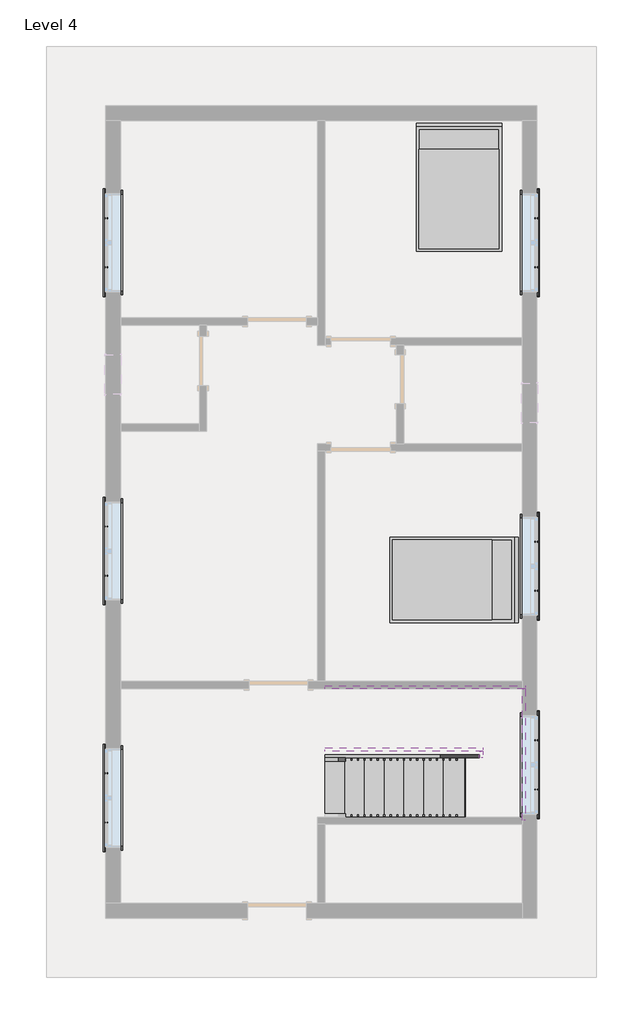
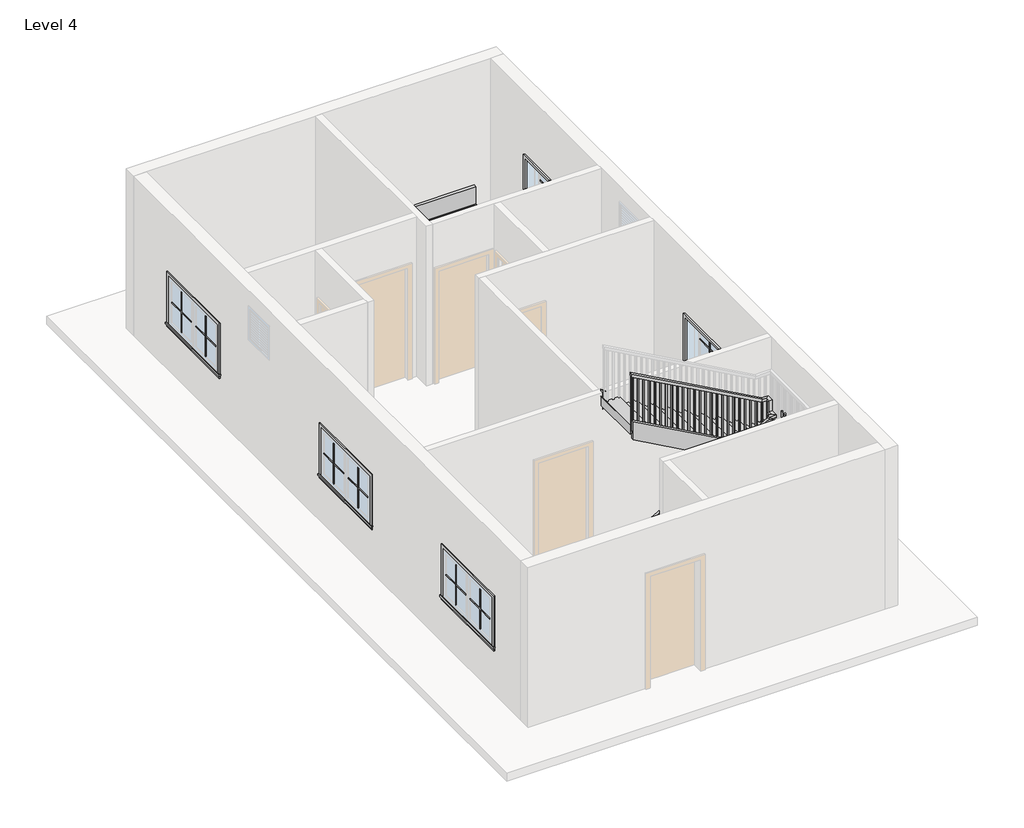
# One storey, part 3 of 3: 24 proxies, 6 members, 2 furniture elements, 1 railing, 1 stair flight.
"""IFC4 building model written with IfcOpenShell, lengths in millimetres."""

from ifc_helpers import new_model, si_unit, frame, origin, place, context, project, spatial, polyline, outline, extrude, faceted_brep, transform, mapped, element, save
from components import muntin_pattern_2x2_muntin_pattern_2x2_9352d081, muntin_pattern_2x2_muntin_pattern_2x2_5c2cbe28, trim_window_exterior_flat_with_sill_979bde60, trim_window_interior_flat_picture_frame_7883d11b, bed_17739_bed_17739_15c61121, stair_flight_ebc403c3

model = new_model("IFC4")

# Units and contexts
model_context = context("Model", 3, world=origin())
ifc_project = project(units=[si_unit("LENGTHUNIT", "METRE", prefix="MILLI")], contexts=[model_context])

# Site, building, storey
site = spatial("IfcSite", under=ifc_project)
building = spatial("IfcBuilding", under=site)
storey = spatial("IfcBuildingStorey", under=building, Name="Level 4", Elevation=9448.8)

# Proxies
placement = place(None, origin())
muntin_pattern_2x2_muntin_pattern_2x2_shape = muntin_pattern_2x2_muntin_pattern_2x2_9352d081(model_context)
element("IfcBuildingElementProxy", 1, Name="Muntin Pattern_2x2 : Muntin Pattern_2x2", ObjectType="Muntin Pattern_2x2 : Muntin Pattern_2x2", at=placement, inside=storey, context=model_context, shape_type="MappedRepresentation", body=[
    mapped(muntin_pattern_2x2_muntin_pattern_2x2_shape, transform((-4579.34688, 3675.02881, 10433.05), x_axis=(0.0, 1.0, 0.0), y_axis=(-1.0, 0.0, 0.0), z_axis=(0.0, 0.0, 1.0))),
])
element("IfcBuildingElementProxy", 2, Name="Muntin Pattern_2x2 : Muntin Pattern_2x2", ObjectType="Muntin Pattern_2x2 : Muntin Pattern_2x2", at=placement, inside=storey, context=model_context, shape_type="MappedRepresentation", body=[
    mapped(muntin_pattern_2x2_muntin_pattern_2x2_shape, transform((-4579.34688, -1087.47119, 10433.05), x_axis=(0.0, 1.0, 0.0), y_axis=(-1.0, 0.0, 0.0), z_axis=(0.0, 0.0, 1.0))),
])
element("IfcBuildingElementProxy", 3, Name="Muntin Pattern_2x2 : Muntin Pattern_2x2", ObjectType="Muntin Pattern_2x2 : Muntin Pattern_2x2", at=placement, inside=storey, context=model_context, shape_type="MappedRepresentation", body=[
    mapped(muntin_pattern_2x2_muntin_pattern_2x2_shape, transform((-4579.34688, -4900.64619, 10433.05), x_axis=(0.0, 1.0, 0.0), y_axis=(-1.0, 0.0, 0.0), z_axis=(0.0, 0.0, 1.0))),
])
element("IfcBuildingElementProxy", 4, Name="Muntin Pattern_2x2 : Muntin Pattern_2x2", ObjectType="Muntin Pattern_2x2 : Muntin Pattern_2x2", at=placement, inside=storey, context=model_context, shape_type="MappedRepresentation", body=[
    mapped(muntin_pattern_2x2_muntin_pattern_2x2_shape, transform((2069.10312, -3630.64619, 10433.05), x_axis=(0.0, -1.0, 0.0), y_axis=(1.0, 0.0, 0.0), z_axis=(0.0, 0.0, 1.0))),
])
element("IfcBuildingElementProxy", 5, Name="Muntin Pattern_2x2 : Muntin Pattern_2x2", ObjectType="Muntin Pattern_2x2 : Muntin Pattern_2x2", at=placement, inside=storey, context=model_context, shape_type="MappedRepresentation", body=[
    mapped(muntin_pattern_2x2_muntin_pattern_2x2_shape, transform((2069.10312, 4433.85381, 10433.05), x_axis=(0.0, -1.0, 0.0), y_axis=(1.0, 0.0, 0.0), z_axis=(0.0, 0.0, 1.0))),
])
element("IfcBuildingElementProxy", 6, Name="Muntin Pattern_2x2 : Muntin Pattern_2x2", ObjectType="Muntin Pattern_2x2 : Muntin Pattern_2x2", at=placement, inside=storey, context=model_context, shape_type="MappedRepresentation", body=[
    mapped(muntin_pattern_2x2_muntin_pattern_2x2_shape, transform((2069.10312, -563.59619, 10433.05), x_axis=(0.0, -1.0, 0.0), y_axis=(1.0, 0.0, 0.0), z_axis=(0.0, 0.0, 1.0))),
])
muntin_pattern_2x2_muntin_pattern_2x2_2_shape = muntin_pattern_2x2_muntin_pattern_2x2_5c2cbe28(model_context)
element("IfcBuildingElementProxy", 7, Name="Muntin Pattern_2x2 : Muntin Pattern_2x2", ObjectType="Muntin Pattern_2x2 : Muntin Pattern_2x2", at=placement, inside=storey, context=model_context, shape_type="MappedRepresentation", body=[
    mapped(muntin_pattern_2x2_muntin_pattern_2x2_2_shape, transform((-4579.34688, 4433.85381, 10433.05), x_axis=(0.0, -1.0, 0.0), y_axis=(1.0, 0.0, 0.0), z_axis=(0.0, 0.0, 1.0))),
])
element("IfcBuildingElementProxy", 8, Name="Muntin Pattern_2x2 : Muntin Pattern_2x2", ObjectType="Muntin Pattern_2x2 : Muntin Pattern_2x2", at=placement, inside=storey, context=model_context, shape_type="MappedRepresentation", body=[
    mapped(muntin_pattern_2x2_muntin_pattern_2x2_2_shape, transform((-4579.34688, -328.64619, 10433.05), x_axis=(0.0, -1.0, 0.0), y_axis=(1.0, 0.0, 0.0), z_axis=(0.0, 0.0, 1.0))),
])
element("IfcBuildingElementProxy", 9, Name="Muntin Pattern_2x2 : Muntin Pattern_2x2", ObjectType="Muntin Pattern_2x2 : Muntin Pattern_2x2", at=placement, inside=storey, context=model_context, shape_type="MappedRepresentation", body=[
    mapped(muntin_pattern_2x2_muntin_pattern_2x2_2_shape, transform((-4579.34688, -4141.82119, 10433.05), x_axis=(0.0, -1.0, 0.0), y_axis=(1.0, 0.0, 0.0), z_axis=(0.0, 0.0, 1.0))),
])
element("IfcBuildingElementProxy", 10, Name="Muntin Pattern_2x2 : Muntin Pattern_2x2", ObjectType="Muntin Pattern_2x2 : Muntin Pattern_2x2", at=placement, inside=storey, context=model_context, shape_type="MappedRepresentation", body=[
    mapped(muntin_pattern_2x2_muntin_pattern_2x2_2_shape, transform((2069.10312, -4389.47119, 10433.05), x_axis=(0.0, 1.0, 0.0), y_axis=(-1.0, 0.0, 0.0), z_axis=(0.0, 0.0, 1.0))),
])
element("IfcBuildingElementProxy", 11, Name="Muntin Pattern_2x2 : Muntin Pattern_2x2", ObjectType="Muntin Pattern_2x2 : Muntin Pattern_2x2", at=placement, inside=storey, context=model_context, shape_type="MappedRepresentation", body=[
    mapped(muntin_pattern_2x2_muntin_pattern_2x2_2_shape, transform((2069.10312, 3675.02881, 10433.05), x_axis=(0.0, 1.0, 0.0), y_axis=(-1.0, 0.0, 0.0), z_axis=(0.0, 0.0, 1.0))),
])
element("IfcBuildingElementProxy", 12, Name="Muntin Pattern_2x2 : Muntin Pattern_2x2", ObjectType="Muntin Pattern_2x2 : Muntin Pattern_2x2", at=placement, inside=storey, context=model_context, shape_type="MappedRepresentation", body=[
    mapped(muntin_pattern_2x2_muntin_pattern_2x2_2_shape, transform((2069.10312, -1322.42119, 10433.05), x_axis=(0.0, 1.0, 0.0), y_axis=(-1.0, 0.0, 0.0), z_axis=(0.0, 0.0, 1.0))),
])
trim_window_exterior_flat_with_sill_shape = trim_window_exterior_flat_with_sill_979bde60(model_context)
element("IfcBuildingElementProxy", 13, Name="Trim-Window-Exterior-Flat : with Sill", ObjectType="Trim-Window-Exterior-Flat : with Sill", at=placement, inside=storey, context=model_context, shape_type="MappedRepresentation", body=[
    mapped(trim_window_exterior_flat_with_sill_shape, transform((-4588.87188, 4054.44131, 11277.6), x_axis=(0.0, -1.0, 0.0), y_axis=(0.0, 0.0, 1.0), z_axis=(-1.0, 0.0, 0.0))),
])
element("IfcBuildingElementProxy", 14, Name="Trim-Window-Exterior-Flat : with Sill", ObjectType="Trim-Window-Exterior-Flat : with Sill", at=placement, inside=storey, context=model_context, shape_type="MappedRepresentation", body=[
    mapped(trim_window_exterior_flat_with_sill_shape, transform((-4588.87188, -708.05869, 11277.6), x_axis=(0.0, -1.0, 0.0), y_axis=(0.0, 0.0, 1.0), z_axis=(-1.0, 0.0, 0.0))),
])
element("IfcBuildingElementProxy", 15, Name="Trim-Window-Exterior-Flat : with Sill", ObjectType="Trim-Window-Exterior-Flat : with Sill", at=placement, inside=storey, context=model_context, shape_type="MappedRepresentation", body=[
    mapped(trim_window_exterior_flat_with_sill_shape, transform((-4588.87188, -4521.23369, 11277.6), x_axis=(0.0, -1.0, 0.0), y_axis=(0.0, 0.0, 1.0), z_axis=(-1.0, 0.0, 0.0))),
])
element("IfcBuildingElementProxy", 16, Name="Trim-Window-Exterior-Flat : with Sill", ObjectType="Trim-Window-Exterior-Flat : with Sill", at=placement, inside=storey, context=model_context, shape_type="MappedRepresentation", body=[
    mapped(trim_window_exterior_flat_with_sill_shape, transform((2078.62812, -4010.05869, 11277.6), x_axis=(0.0, 1.0, 0.0), y_axis=(0.0, 0.0, 1.0), z_axis=(1.0, 0.0, 0.0))),
])
element("IfcBuildingElementProxy", 17, Name="Trim-Window-Exterior-Flat : with Sill", ObjectType="Trim-Window-Exterior-Flat : with Sill", at=placement, inside=storey, context=model_context, shape_type="MappedRepresentation", body=[
    mapped(trim_window_exterior_flat_with_sill_shape, transform((2078.62812, 4054.44131, 11277.6), x_axis=(0.0, 1.0, 0.0), y_axis=(0.0, 0.0, 1.0), z_axis=(1.0, 0.0, 0.0))),
])
element("IfcBuildingElementProxy", 18, Name="Trim-Window-Exterior-Flat : with Sill", ObjectType="Trim-Window-Exterior-Flat : with Sill", at=placement, inside=storey, context=model_context, shape_type="MappedRepresentation", body=[
    mapped(trim_window_exterior_flat_with_sill_shape, transform((2078.62812, -943.00869, 11277.6), x_axis=(0.0, 1.0, 0.0), y_axis=(0.0, 0.0, 1.0), z_axis=(1.0, 0.0, 0.0))),
])
trim_window_interior_flat_picture_frame_shape = trim_window_interior_flat_picture_frame_7883d11b(model_context)
element("IfcBuildingElementProxy", 19, Name="Trim-Window-Interior-Flat : Picture Frame", ObjectType="Trim-Window-Interior-Flat : Picture Frame", at=placement, inside=storey, context=model_context, shape_type="MappedRepresentation", body=[
    mapped(trim_window_interior_flat_picture_frame_shape, transform((-4360.27188, 4054.44131, 11277.6), x_axis=(0.0, 1.0, 0.0), y_axis=(0.0, 0.0, 1.0), z_axis=(1.0, 0.0, 0.0))),
])
element("IfcBuildingElementProxy", 20, Name="Trim-Window-Interior-Flat : Picture Frame", ObjectType="Trim-Window-Interior-Flat : Picture Frame", at=placement, inside=storey, context=model_context, shape_type="MappedRepresentation", body=[
    mapped(trim_window_interior_flat_picture_frame_shape, transform((-4360.27188, -708.05869, 11277.6), x_axis=(0.0, 1.0, 0.0), y_axis=(0.0, 0.0, 1.0), z_axis=(1.0, 0.0, 0.0))),
])
element("IfcBuildingElementProxy", 21, Name="Trim-Window-Interior-Flat : Picture Frame", ObjectType="Trim-Window-Interior-Flat : Picture Frame", at=placement, inside=storey, context=model_context, shape_type="MappedRepresentation", body=[
    mapped(trim_window_interior_flat_picture_frame_shape, transform((-4360.27188, -4521.23369, 11277.6), x_axis=(0.0, 1.0, 0.0), y_axis=(0.0, 0.0, 1.0), z_axis=(1.0, 0.0, 0.0))),
])
element("IfcBuildingElementProxy", 22, Name="Trim-Window-Interior-Flat : Picture Frame", ObjectType="Trim-Window-Interior-Flat : Picture Frame", at=placement, inside=storey, context=model_context, shape_type="MappedRepresentation", body=[
    mapped(trim_window_interior_flat_picture_frame_shape, transform((1850.02812, -4010.05869, 11277.6), x_axis=(0.0, -1.0, 0.0), y_axis=(0.0, 0.0, 1.0), z_axis=(-1.0, 0.0, 0.0))),
])
element("IfcBuildingElementProxy", 23, Name="Trim-Window-Interior-Flat : Picture Frame", ObjectType="Trim-Window-Interior-Flat : Picture Frame", at=placement, inside=storey, context=model_context, shape_type="MappedRepresentation", body=[
    mapped(trim_window_interior_flat_picture_frame_shape, transform((1850.02812, 4054.44131, 11277.6), x_axis=(0.0, -1.0, 0.0), y_axis=(0.0, 0.0, 1.0), z_axis=(-1.0, 0.0, 0.0))),
])
element("IfcBuildingElementProxy", 24, Name="Trim-Window-Interior-Flat : Picture Frame", ObjectType="Trim-Window-Interior-Flat : Picture Frame", at=placement, inside=storey, context=model_context, shape_type="MappedRepresentation", body=[
    mapped(trim_window_interior_flat_picture_frame_shape, transform((1850.02812, -943.00869, 11277.6), x_axis=(0.0, -1.0, 0.0), y_axis=(0.0, 0.0, 1.0), z_axis=(-1.0, 0.0, 0.0))),
])

# Furniture
bed_17739_bed_17739_shape = bed_17739_bed_17739_15c61121(model_context)
element("IfcFurniture", 25, ObjectType="Bed_17739 : Bed_17739", at=placement, inside=storey, context=model_context, shape_type="MappedRepresentation", body=[
    mapped(bed_17739_bed_17739_shape, transform((872.12812, 4886.29131, 9448.8), x_axis=(1.0, 0.0, 0.0), y_axis=(0.0, 1.0, 0.0), z_axis=(0.0, 0.0, 1.0))),
])
element("IfcFurniture", 26, ObjectType="Bed_17739 : Bed_17739", at=placement, inside=storey, context=model_context, shape_type="MappedRepresentation", body=[
    mapped(bed_17739_bed_17739_shape, transform((770.52812, -1152.55869, 9448.8), x_axis=(0.0, -1.0, 0.0), y_axis=(1.0, 0.0, 0.0), z_axis=(0.0, 0.0, 1.0))),
])

# Members
element("IfcMember", 27, ObjectType="Stringer - 2\" Width", at=placement, inside=storey, context=model_context, shape_type="SweptSolid", body=[
    extrude(outline(polyline([(9656.3983948, -1197.97188), (9448.8, -1197.97188), (9448.8, -944.0273772), (10634.1641651, 1189.62812), (10982.8428392, 1189.62812), (9656.3983948, -1197.97188)])), frame((0.0, -3902.10869, 0.0), z_axis=(0.0, 1.0, 0.0), x_axis=(0.0, 0.0, 1.0)), (0.0, 0.0, 1.0), 50.8),
])
element("IfcMember", 28, ObjectType="Stringer - 2\" Width", at=placement, inside=storey, context=model_context, shape_type="SweptSolid", body=[
    extrude(outline(polyline([(1240.42812, -3902.10869), (1189.62812, -3902.10869), (1189.62812, -3800.50869), (1240.42812, -3800.50869), (1240.42812, -3902.10869)])), frame((0.0, 0.0, 10744.2), z_axis=(0.0, 0.0, 1.0), x_axis=(1.0, 0.0, 0.0)), (0.0, 0.0, 1.0), 304.8),
])
element("IfcMember", 29, ObjectType="Stringer - 2\" Width", at=placement, inside=storey, context=model_context, shape_type="SweptSolid", body=[
    extrude(outline(polyline([(10831.7197207, 1240.42812), (11180.3983948, 1240.42812), (12535.0650614, -1197.97188), (12186.3863873, -1197.97188), (10831.7197207, 1240.42812)])), frame((0.0, -3800.50869, 0.0), z_axis=(0.0, 1.0, 0.0), x_axis=(0.0, 0.0, 1.0)), (0.0, 0.0, 1.0), 50.8),
])
element("IfcMember", 30, ObjectType="Stringer - 2\" Width", at=placement, inside=storey, context=model_context, shape_type="SweptSolid", body=[
    extrude(outline(polyline([(9656.3983948, -1197.97188), (9448.8, -1197.97188), (9448.8, -944.0273772), (11001.053054, 1850.02812), (11049.0, 1850.02812), (11049.0, 1308.7110094), (9656.3983948, -1197.97188)])), frame((0.0, -4867.30869, 0.0), z_axis=(0.0, 1.0, 0.0), x_axis=(0.0, 0.0, 1.0)), (0.0, 0.0, 1.0), 50.8),
])
element("IfcMember", 31, ObjectType="Stringer - 2\" Width", at=placement, inside=storey, context=model_context, shape_type="SweptSolid", body=[
    extrude(outline(polyline([(1900.82812, -4867.30869), (1850.02812, -4867.30869), (1850.02812, -2835.30869), (1900.82812, -2835.30869), (1900.82812, -4867.30869)])), frame((0.0, 0.0, 10744.2), z_axis=(0.0, 0.0, 1.0), x_axis=(1.0, 0.0, 0.0)), (0.0, 0.0, 1.0), 304.8),
])
element("IfcMember", 32, ObjectType="Stringer - 2\" Width", at=placement, inside=storey, context=model_context, shape_type="SweptSolid", body=[
    extrude(outline(polyline([(10744.2, 1900.82812), (10813.5095059, 1900.82812), (12535.0650614, -1197.97188), (12186.3863873, -1197.97188), (10744.2, 1397.9636172), (10744.2, 1900.82812)])), frame((0.0, -2835.30869, 0.0), z_axis=(0.0, 1.0, 0.0), x_axis=(0.0, 0.0, 1.0)), (0.0, 0.0, 1.0), 50.8),
])

# Railing
element("IfcRailing", 33, ObjectType="Handrail - Rectangular", at=placement, inside=storey, context=model_context, shape_type="SolidModel", body=[
    faceted_brep([(-1197.97188, -3902.10869, 10532.5333333), (-1197.97188, -3902.10869, 10474.420221), (-1197.97188, -3952.90869, 10474.420221), (-1197.97188, -3952.90869, 10532.5333333), (1164.22812, -3902.10869, 11844.8666667), (1215.02812, -3902.10869, 11814.9757765), (1215.02812, -3952.90869, 11814.9757765), (1164.22812, -3952.90869, 11844.8666667), (1164.22812, -3902.10869, 11887.2), (1215.02812, -3902.10869, 11836.4), (1215.02812, -3952.90869, 11836.4), (1164.22812, -3952.90869, 11887.2), (1240.42812, -3902.10869, 11887.2), (1240.42812, -3902.10869, 11836.4), (1291.22812, -3952.90869, 11836.4), (1291.22812, -3952.90869, 11887.2), (1240.42812, -3825.90869, 11887.2), (1240.42812, -3775.10869, 11836.4), (1291.22812, -3775.10869, 11836.4), (1291.22812, -3825.90869, 11887.2), (1240.42812, -3825.90869, 12098.8666667), (1240.42812, -3775.10869, 12048.0666667), (1291.22812, -3775.10869, 12048.0666667), (1291.22812, -3825.90869, 12098.8666667), (1240.42812, -3749.70869, 12098.8666667), (1240.42812, -3749.70869, 12048.0666667), (1291.22812, -3698.90869, 12048.0666667), (1291.22812, -3698.90869, 12098.8666667), (1164.22812, -3749.70869, 12098.8666667), (1151.0645177, -3749.70869, 12048.0666667), (1151.0645177, -3698.90869, 12048.0666667), (1164.22812, -3698.90869, 12098.8666667), (-1197.97188, -3749.70869, 13411.2), (-1197.97188, -3698.90869, 13411.2), (-1197.97188, -3698.90869, 13353.0868876), (-1197.97188, -3749.70869, 13353.0868876)], [[[0, 1, 2, 3]], [[1, 0, 4, 5]], [[2, 1, 5, 6]], [[3, 2, 6, 7]], [[0, 3, 7, 4]], [[5, 4, 8, 9]], [[6, 5, 9, 10]], [[7, 6, 10, 11]], [[4, 7, 11, 8]], [[9, 8, 12, 13]], [[10, 9, 13, 14]], [[11, 10, 14, 15]], [[8, 11, 15, 12]], [[13, 12, 16, 17]], [[14, 13, 17, 18]], [[15, 14, 18, 19]], [[12, 15, 19, 16]], [[17, 16, 20, 21]], [[18, 17, 21, 22]], [[19, 18, 22, 23]], [[16, 19, 23, 20]], [[21, 20, 24, 25]], [[22, 21, 25, 26]], [[23, 22, 26, 27]], [[20, 23, 27, 24]], [[25, 24, 28, 29]], [[26, 25, 29, 30]], [[27, 26, 30, 31]], [[24, 27, 31, 28]], [[32, 33, 34, 35]], [[29, 28, 32, 35]], [[30, 29, 35, 34]], [[31, 30, 34, 33]], [[28, 31, 33, 32]]]),
    extrude(outline(polyline([(13344.2674432, -1182.09688), (12327.4666667, -1182.09688), (12327.4666667, -1163.04688), (13333.6841099, -1163.04688), (13344.2674432, -1182.09688)])), frame((0.0, -3733.83369, 0.0), z_axis=(0.0, 1.0, 0.0), x_axis=(0.0, 0.0, 1.0)), (0.0, 0.0, 1.0), 19.05),
    extrude(outline(polyline([(13287.8229988, -1080.49688), (12327.4666667, -1080.49688), (12327.4666667, -1061.44688), (13277.2396654, -1061.44688), (13287.8229988, -1080.49688)])), frame((0.0, -3733.83369, 0.0), z_axis=(0.0, 1.0, 0.0), x_axis=(0.0, 0.0, 1.0)), (0.0, 0.0, 1.0), 19.05),
    extrude(outline(polyline([(13231.3785543, -978.89688), (12327.4666667, -978.89688), (12327.4666667, -959.84688), (13220.795221, -959.84688), (13231.3785543, -978.89688)])), frame((0.0, -3733.83369, 0.0), z_axis=(0.0, 1.0, 0.0), x_axis=(0.0, 0.0, 1.0)), (0.0, 0.0, 1.0), 19.05),
    extrude(outline(polyline([(13174.9341099, -877.29688), (12158.1333333, -877.29688), (12158.1333333, -858.24688), (13164.3507765, -858.24688), (13174.9341099, -877.29688)])), frame((0.0, -3733.83369, 0.0), z_axis=(0.0, 1.0, 0.0), x_axis=(0.0, 0.0, 1.0)), (0.0, 0.0, 1.0), 19.05),
    extrude(outline(polyline([(13118.4896654, -775.69688), (12158.1333333, -775.69688), (12158.1333333, -756.64688), (13107.9063321, -756.64688), (13118.4896654, -775.69688)])), frame((0.0, -3733.83369, 0.0), z_axis=(0.0, 1.0, 0.0), x_axis=(0.0, 0.0, 1.0)), (0.0, 0.0, 1.0), 19.05),
    extrude(outline(polyline([(13062.045221, -674.09688), (12158.1333333, -674.09688), (12158.1333333, -655.04688), (13051.4618876, -655.04688), (13062.045221, -674.09688)])), frame((0.0, -3733.83369, 0.0), z_axis=(0.0, 1.0, 0.0), x_axis=(0.0, 0.0, 1.0)), (0.0, 0.0, 1.0), 19.05),
    extrude(outline(polyline([(13005.6007765, -572.49688), (11988.8, -572.49688), (11988.8, -553.44688), (12995.0174432, -553.44688), (13005.6007765, -572.49688)])), frame((0.0, -3733.83369, 0.0), z_axis=(0.0, 1.0, 0.0), x_axis=(0.0, 0.0, 1.0)), (0.0, 0.0, 1.0), 19.05),
    extrude(outline(polyline([(12949.1563321, -470.89688), (11988.8, -470.89688), (11988.8, -451.84688), (12938.5729988, -451.84688), (12949.1563321, -470.89688)])), frame((0.0, -3733.83369, 0.0), z_axis=(0.0, 1.0, 0.0), x_axis=(0.0, 0.0, 1.0)), (0.0, 0.0, 1.0), 19.05),
    extrude(outline(polyline([(12892.7118876, -369.29688), (11988.8, -369.29688), (11988.8, -350.24688), (12882.1285543, -350.24688), (12892.7118876, -369.29688)])), frame((0.0, -3733.83369, 0.0), z_axis=(0.0, 1.0, 0.0), x_axis=(0.0, 0.0, 1.0)), (0.0, 0.0, 1.0), 19.05),
    extrude(outline(polyline([(12836.2674432, -267.69688), (11819.4666667, -267.69688), (11819.4666667, -248.64688), (12825.6841099, -248.64688), (12836.2674432, -267.69688)])), frame((0.0, -3733.83369, 0.0), z_axis=(0.0, 1.0, 0.0), x_axis=(0.0, 0.0, 1.0)), (0.0, 0.0, 1.0), 19.05),
    extrude(outline(polyline([(12779.8229988, -166.09688), (11819.4666667, -166.09688), (11819.4666667, -147.04688), (12769.2396654, -147.04688), (12779.8229988, -166.09688)])), frame((0.0, -3733.83369, 0.0), z_axis=(0.0, 1.0, 0.0), x_axis=(0.0, 0.0, 1.0)), (0.0, 0.0, 1.0), 19.05),
    extrude(outline(polyline([(12723.3785543, -64.49688), (11819.4666667, -64.49688), (11819.4666667, -45.44688), (12712.795221, -45.44688), (12723.3785543, -64.49688)])), frame((0.0, -3733.83369, 0.0), z_axis=(0.0, 1.0, 0.0), x_axis=(0.0, 0.0, 1.0)), (0.0, 0.0, 1.0), 19.05),
    extrude(outline(polyline([(12666.9341099, 37.10312), (11650.1333333, 37.10312), (11650.1333333, 56.15312), (12656.3507765, 56.15312), (12666.9341099, 37.10312)])), frame((0.0, -3733.83369, 0.0), z_axis=(0.0, 1.0, 0.0), x_axis=(0.0, 0.0, 1.0)), (0.0, 0.0, 1.0), 19.05),
    extrude(outline(polyline([(12610.4896654, 138.70312), (11650.1333333, 138.70312), (11650.1333333, 157.75312), (12599.9063321, 157.75312), (12610.4896654, 138.70312)])), frame((0.0, -3733.83369, 0.0), z_axis=(0.0, 1.0, 0.0), x_axis=(0.0, 0.0, 1.0)), (0.0, 0.0, 1.0), 19.05),
    extrude(outline(polyline([(12554.045221, 240.30312), (11650.1333333, 240.30312), (11650.1333333, 259.35312), (12543.4618876, 259.35312), (12554.045221, 240.30312)])), frame((0.0, -3733.83369, 0.0), z_axis=(0.0, 1.0, 0.0), x_axis=(0.0, 0.0, 1.0)), (0.0, 0.0, 1.0), 19.05),
    extrude(outline(polyline([(12497.6007765, 341.90312), (11480.8, 341.90312), (11480.8, 360.95312), (12487.0174432, 360.95312), (12497.6007765, 341.90312)])), frame((0.0, -3733.83369, 0.0), z_axis=(0.0, 1.0, 0.0), x_axis=(0.0, 0.0, 1.0)), (0.0, 0.0, 1.0), 19.05),
    extrude(outline(polyline([(12441.1563321, 443.50312), (11480.8, 443.50312), (11480.8, 462.55312), (12430.5729988, 462.55312), (12441.1563321, 443.50312)])), frame((0.0, -3733.83369, 0.0), z_axis=(0.0, 1.0, 0.0), x_axis=(0.0, 0.0, 1.0)), (0.0, 0.0, 1.0), 19.05),
    extrude(outline(polyline([(12384.7118876, 545.10312), (11480.8, 545.10312), (11480.8, 564.15312), (12374.1285543, 564.15312), (12384.7118876, 545.10312)])), frame((0.0, -3733.83369, 0.0), z_axis=(0.0, 1.0, 0.0), x_axis=(0.0, 0.0, 1.0)), (0.0, 0.0, 1.0), 19.05),
    extrude(outline(polyline([(12328.2674432, 646.70312), (11311.4666667, 646.70312), (11311.4666667, 665.75312), (12317.6841099, 665.75312), (12328.2674432, 646.70312)])), frame((0.0, -3733.83369, 0.0), z_axis=(0.0, 1.0, 0.0), x_axis=(0.0, 0.0, 1.0)), (0.0, 0.0, 1.0), 19.05),
    extrude(outline(polyline([(12271.8229988, 748.30312), (11311.4666667, 748.30312), (11311.4666667, 767.35312), (12261.2396654, 767.35312), (12271.8229988, 748.30312)])), frame((0.0, -3733.83369, 0.0), z_axis=(0.0, 1.0, 0.0), x_axis=(0.0, 0.0, 1.0)), (0.0, 0.0, 1.0), 19.05),
    extrude(outline(polyline([(12215.3785543, 849.90312), (11311.4666667, 849.90312), (11311.4666667, 868.95312), (12204.795221, 868.95312), (12215.3785543, 849.90312)])), frame((0.0, -3733.83369, 0.0), z_axis=(0.0, 1.0, 0.0), x_axis=(0.0, 0.0, 1.0)), (0.0, 0.0, 1.0), 19.05),
    extrude(outline(polyline([(12158.9341099, 951.50312), (11142.1333333, 951.50312), (11142.1333333, 970.55312), (12148.3507765, 970.55312), (12158.9341099, 951.50312)])), frame((0.0, -3733.83369, 0.0), z_axis=(0.0, 1.0, 0.0), x_axis=(0.0, 0.0, 1.0)), (0.0, 0.0, 1.0), 19.05),
    extrude(outline(polyline([(12102.4896654, 1053.10312), (11142.1333333, 1053.10312), (11142.1333333, 1072.15312), (12091.9063321, 1072.15312), (12102.4896654, 1053.10312)])), frame((0.0, -3733.83369, 0.0), z_axis=(0.0, 1.0, 0.0), x_axis=(0.0, 0.0, 1.0)), (0.0, 0.0, 1.0), 19.05),
    extrude(outline(polyline([(12046.045221, 1154.70312), (11142.1333333, 1154.70312), (11142.1333333, 1173.75312), (12035.4618876, 1173.75312), (12046.045221, 1154.70312)])), frame((0.0, -3733.83369, 0.0), z_axis=(0.0, 1.0, 0.0), x_axis=(0.0, 0.0, 1.0)), (0.0, 0.0, 1.0), 19.05),
    extrude(outline(polyline([(1256.30312, -3835.43369), (1256.30312, -3816.38369), (1275.35312, -3816.38369), (1275.35312, -3835.43369), (1256.30312, -3835.43369)])), frame((0.0, 0.0, 10972.8), z_axis=(0.0, 0.0, 1.0), x_axis=(1.0, 0.0, 0.0)), (0.0, 0.0, 1.0), 863.6),
    extrude(outline(polyline([(1230.90312, -3917.98369), (1249.95312, -3917.98369), (1249.95312, -3937.03369), (1230.90312, -3937.03369), (1230.90312, -3917.98369)])), frame((0.0, 0.0, 10972.8), z_axis=(0.0, 0.0, 1.0), x_axis=(1.0, 0.0, 0.0)), (0.0, 0.0, 1.0), 863.6),
    extrude(outline(polyline([(11767.3507765, 1129.30312), (10803.4666667, 1129.30312), (10803.4666667, 1148.35312), (11777.9341099, 1148.35312), (11767.3507765, 1129.30312)])), frame((0.0, -3937.03369, 0.0), z_axis=(0.0, 1.0, 0.0), x_axis=(0.0, 0.0, 1.0)), (0.0, 0.0, 1.0), 19.05),
    extrude(outline(polyline([(11710.9063321, 1027.70312), (10803.4666667, 1027.70312), (10803.4666667, 1046.75312), (11721.4896654, 1046.75312), (11710.9063321, 1027.70312)])), frame((0.0, -3937.03369, 0.0), z_axis=(0.0, 1.0, 0.0), x_axis=(0.0, 0.0, 1.0)), (0.0, 0.0, 1.0), 19.05),
    extrude(outline(polyline([(11654.4618876, 926.10312), (10803.4666667, 926.10312), (10803.4666667, 945.15312), (11665.045221, 945.15312), (11654.4618876, 926.10312)])), frame((0.0, -3937.03369, 0.0), z_axis=(0.0, 1.0, 0.0), x_axis=(0.0, 0.0, 1.0)), (0.0, 0.0, 1.0), 19.05),
    extrude(outline(polyline([(11598.0174432, 824.50312), (10634.1333333, 824.50312), (10634.1333333, 843.55312), (11608.6007765, 843.55312), (11598.0174432, 824.50312)])), frame((0.0, -3937.03369, 0.0), z_axis=(0.0, 1.0, 0.0), x_axis=(0.0, 0.0, 1.0)), (0.0, 0.0, 1.0), 19.05),
    extrude(outline(polyline([(11541.5729988, 722.90312), (10634.1333333, 722.90312), (10634.1333333, 741.95312), (11552.1563321, 741.95312), (11541.5729988, 722.90312)])), frame((0.0, -3937.03369, 0.0), z_axis=(0.0, 1.0, 0.0), x_axis=(0.0, 0.0, 1.0)), (0.0, 0.0, 1.0), 19.05),
    extrude(outline(polyline([(11485.1285543, 621.30312), (10634.1333333, 621.30312), (10634.1333333, 640.35312), (11495.7118876, 640.35312), (11485.1285543, 621.30312)])), frame((0.0, -3937.03369, 0.0), z_axis=(0.0, 1.0, 0.0), x_axis=(0.0, 0.0, 1.0)), (0.0, 0.0, 1.0), 19.05),
    extrude(outline(polyline([(11428.6841099, 519.70312), (10464.8, 519.70312), (10464.8, 538.75312), (11439.2674432, 538.75312), (11428.6841099, 519.70312)])), frame((0.0, -3937.03369, 0.0), z_axis=(0.0, 1.0, 0.0), x_axis=(0.0, 0.0, 1.0)), (0.0, 0.0, 1.0), 19.05),
    extrude(outline(polyline([(11372.2396654, 418.10312), (10464.8, 418.10312), (10464.8, 437.15312), (11382.8229988, 437.15312), (11372.2396654, 418.10312)])), frame((0.0, -3937.03369, 0.0), z_axis=(0.0, 1.0, 0.0), x_axis=(0.0, 0.0, 1.0)), (0.0, 0.0, 1.0), 19.05),
    extrude(outline(polyline([(11315.795221, 316.50312), (10464.8, 316.50312), (10464.8, 335.55312), (11326.3785543, 335.55312), (11315.795221, 316.50312)])), frame((0.0, -3937.03369, 0.0), z_axis=(0.0, 1.0, 0.0), x_axis=(0.0, 0.0, 1.0)), (0.0, 0.0, 1.0), 19.05),
    extrude(outline(polyline([(11259.3507765, 214.90312), (10295.4666667, 214.90312), (10295.4666667, 233.95312), (11269.9341099, 233.95312), (11259.3507765, 214.90312)])), frame((0.0, -3937.03369, 0.0), z_axis=(0.0, 1.0, 0.0), x_axis=(0.0, 0.0, 1.0)), (0.0, 0.0, 1.0), 19.05),
    extrude(outline(polyline([(11202.9063321, 113.30312), (10295.4666667, 113.30312), (10295.4666667, 132.35312), (11213.4896654, 132.35312), (11202.9063321, 113.30312)])), frame((0.0, -3937.03369, 0.0), z_axis=(0.0, 1.0, 0.0), x_axis=(0.0, 0.0, 1.0)), (0.0, 0.0, 1.0), 19.05),
    extrude(outline(polyline([(11146.4618876, 11.70312), (10295.4666667, 11.70312), (10295.4666667, 30.75312), (11157.045221, 30.75312), (11146.4618876, 11.70312)])), frame((0.0, -3937.03369, 0.0), z_axis=(0.0, 1.0, 0.0), x_axis=(0.0, 0.0, 1.0)), (0.0, 0.0, 1.0), 19.05),
    extrude(outline(polyline([(11090.0174432, -89.89688), (10126.1333333, -89.89688), (10126.1333333, -70.84688), (11100.6007765, -70.84688), (11090.0174432, -89.89688)])), frame((0.0, -3937.03369, 0.0), z_axis=(0.0, 1.0, 0.0), x_axis=(0.0, 0.0, 1.0)), (0.0, 0.0, 1.0), 19.05),
    extrude(outline(polyline([(11033.5729988, -191.49688), (10126.1333333, -191.49688), (10126.1333333, -172.44688), (11044.1563321, -172.44688), (11033.5729988, -191.49688)])), frame((0.0, -3937.03369, 0.0), z_axis=(0.0, 1.0, 0.0), x_axis=(0.0, 0.0, 1.0)), (0.0, 0.0, 1.0), 19.05),
    extrude(outline(polyline([(10977.1285543, -293.09688), (10126.1333333, -293.09688), (10126.1333333, -274.04688), (10987.7118876, -274.04688), (10977.1285543, -293.09688)])), frame((0.0, -3937.03369, 0.0), z_axis=(0.0, 1.0, 0.0), x_axis=(0.0, 0.0, 1.0)), (0.0, 0.0, 1.0), 19.05),
    extrude(outline(polyline([(10920.6841099, -394.69688), (9956.8, -394.69688), (9956.8, -375.64688), (10931.2674432, -375.64688), (10920.6841099, -394.69688)])), frame((0.0, -3937.03369, 0.0), z_axis=(0.0, 1.0, 0.0), x_axis=(0.0, 0.0, 1.0)), (0.0, 0.0, 1.0), 19.05),
    extrude(outline(polyline([(10864.2396654, -496.29688), (9956.8, -496.29688), (9956.8, -477.24688), (10874.8229988, -477.24688), (10864.2396654, -496.29688)])), frame((0.0, -3937.03369, 0.0), z_axis=(0.0, 1.0, 0.0), x_axis=(0.0, 0.0, 1.0)), (0.0, 0.0, 1.0), 19.05),
    extrude(outline(polyline([(10807.795221, -597.89688), (9956.8, -597.89688), (9956.8, -578.84688), (10818.3785543, -578.84688), (10807.795221, -597.89688)])), frame((0.0, -3937.03369, 0.0), z_axis=(0.0, 1.0, 0.0), x_axis=(0.0, 0.0, 1.0)), (0.0, 0.0, 1.0), 19.05),
    extrude(outline(polyline([(10751.3507765, -699.49688), (9787.4666667, -699.49688), (9787.4666667, -680.44688), (10761.9341099, -680.44688), (10751.3507765, -699.49688)])), frame((0.0, -3937.03369, 0.0), z_axis=(0.0, 1.0, 0.0), x_axis=(0.0, 0.0, 1.0)), (0.0, 0.0, 1.0), 19.05),
    extrude(outline(polyline([(10694.9063321, -801.09688), (9787.4666667, -801.09688), (9787.4666667, -782.04688), (10705.4896654, -782.04688), (10694.9063321, -801.09688)])), frame((0.0, -3937.03369, 0.0), z_axis=(0.0, 1.0, 0.0), x_axis=(0.0, 0.0, 1.0)), (0.0, 0.0, 1.0), 19.05),
    extrude(outline(polyline([(10638.4618876, -902.69688), (9787.4666667, -902.69688), (9787.4666667, -883.64688), (10649.045221, -883.64688), (10638.4618876, -902.69688)])), frame((0.0, -3937.03369, 0.0), z_axis=(0.0, 1.0, 0.0), x_axis=(0.0, 0.0, 1.0)), (0.0, 0.0, 1.0), 19.05),
    extrude(outline(polyline([(10582.0174432, -1004.29688), (9618.1333333, -1004.29688), (9618.1333333, -985.24688), (10592.6007765, -985.24688), (10582.0174432, -1004.29688)])), frame((0.0, -3937.03369, 0.0), z_axis=(0.0, 1.0, 0.0), x_axis=(0.0, 0.0, 1.0)), (0.0, 0.0, 1.0), 19.05),
    extrude(outline(polyline([(10525.5729988, -1105.89688), (9618.1333333, -1105.89688), (9618.1333333, -1086.84688), (10536.1563321, -1086.84688), (10525.5729988, -1105.89688)])), frame((0.0, -3937.03369, 0.0), z_axis=(0.0, 1.0, 0.0), x_axis=(0.0, 0.0, 1.0)), (0.0, 0.0, 1.0), 19.05),
    extrude(outline(polyline([(1256.30312, -3733.83369), (1256.30312, -3714.78369), (1275.35312, -3714.78369), (1275.35312, -3733.83369), (1256.30312, -3733.83369)])), frame((0.0, 0.0, 10972.8), z_axis=(0.0, 0.0, 1.0), x_axis=(1.0, 0.0, 0.0)), (0.0, 0.0, 1.0), 1075.2666667),
    extrude(outline(polyline([(1256.30312, -3917.98369), (1275.35312, -3917.98369), (1275.35312, -3937.03369), (1256.30312, -3937.03369), (1256.30312, -3917.98369)])), frame((0.0, 0.0, 10972.8), z_axis=(0.0, 0.0, 1.0), x_axis=(1.0, 0.0, 0.0)), (0.0, 0.0, 1.0), 863.6),
    extrude(outline(polyline([(13353.0868876, -1197.97188), (12327.4666667, -1197.97188), (12327.4666667, -1178.92188), (13342.5035543, -1178.92188), (13353.0868876, -1197.97188)])), frame((0.0, -3733.83369, 0.0), z_axis=(0.0, 1.0, 0.0), x_axis=(0.0, 0.0, 1.0)), (0.0, 0.0, 1.0), 19.05),
    extrude(outline(polyline([(10474.420221, -1197.97188), (9618.1333333, -1197.97188), (9618.1333333, -1178.92188), (10485.0035543, -1178.92188), (10474.420221, -1197.97188)])), frame((0.0, -3937.03369, 0.0), z_axis=(0.0, 1.0, 0.0), x_axis=(0.0, 0.0, 1.0)), (0.0, 0.0, 1.0), 19.05),
])

# Stair flight
stair_flight_shape = stair_flight_ebc403c3(model_context)
element("IfcStairFlight", 34, ObjectType="2\" Tread 1\" Nosing 1/4\" Riser", at=placement, inside=storey, context=model_context, shape_type="MappedRepresentation", body=[
    mapped(stair_flight_shape, transform((0.0, 0.0, 0.0), x_axis=(1.0, 0.0, 0.0), y_axis=(0.0, 1.0, 0.0), z_axis=(0.0, 0.0, 1.0))),
])

save(model, "model.ifc")

# Revit data of these elements
# Type "Muntin Pattern_2x2 : Muntin Pattern_2x2"
#   Width [instance default] = 4' - 0"
#   Thickness = 0' - 0 1/2"
#   Height [instance default] = 4' - 0"
#   Distance = 0' - 0 3/4"
#   Interior Material [instance default] = none
#   Exterior Material [instance default] = none
#   Default Elevation = 0
# Type "Trim-Window-Exterior-Flat : with Sill"
#   Trim Width = 0' - 2 1/4"
#   Trim Thickness_Picture Frame = 0' - 1 1/4"
#   Trim Thickness_with Sill = 0' - 0 3/4"
#   Sill Thickness = 0' - 1 1/4"
#   Opening Width [instance default] = 2' - 0"
#   Opening Height [instance default] = 3' - 0"
#   Default Elevation = 4' - 0"
#   Sill = yes
#   Picture Frame = no
#   Trim Material [instance default] = none
# Type "Trim-Window-Interior-Flat : Picture Frame"
#   Trim Thickness_Picture Frame = 0' - 1 1/4"
#   Trim Width = 0' - 2 1/4"
#   Trim Thickness_with Sill = 0' - 0 3/4"
#   Sill Thickness = 0' - 1 1/4"
#   Opening Width [instance default] = 2' - 0"
#   Opening Height [instance default] = 3' - 0"
#   Default Elevation = 4' - 0"
#   Sill = no
#   Picture Frame = yes
#   Trim Material [instance default] = none
# Type "Bed_17739 : Bed_17739"
#   Default Elevation = 0
# Type "Handrail - Rectangular"
#   Assembly Code = "C2010400"
#   built-in parameter 1008612 = 0.0416667 (stored number, unit not read)
#   built-in parameter 1008611 = 0.0416667 (stored number, unit not read)
#   built-in parameter 1008609 = 0.333333 (stored number, unit not read)
#   built-in parameter 1008604 = 0.166667 (stored number, unit not read)
#   built-in parameter 1008603 = 0.166667 (stored number, unit not read)
#   Railing Height = 3' - 0"
#   built-in parameter 1008630 = 2
#   built-in parameter 1008610 = 2
#   built-in parameter 1008618 = Baluster - Square : 3/4"
# Elements 1, 2, 3, 4, 5, 6, 7, 8, 9, 10, 11, 12 (IfcBuildingElementProxy, "Muntin Pattern_2x2 : Muntin Pattern_2x2")
#   Width = 2' - 0 5/8"
#   Height = 2' - 6 1/2"
#   Interior Material = Wood - Stained
#   Exterior Material = Clad - White
#   Phase Created = New Construction
#   Materials on its faces: "Clad - White", "Wood - Stained"
# Elements 13, 14, 15, 16, 17, 18 (IfcBuildingElementProxy, "Trim-Window-Exterior-Flat : with Sill")
#   Opening Width = 5' - 0"
#   Opening Height = 3' - 0"
#   Trim Material = Clad - White
#   Phase Created = New Construction
#   Materials on its faces: "Clad - White"
# Elements 19, 20, 21, 22, 23, 24 (IfcBuildingElementProxy, "Trim-Window-Interior-Flat : Picture Frame")
#   Opening Width = 5' - 0"
#   Opening Height = 3' - 0"
#   Trim Material = Wood - Stained
#   Phase Created = New Construction
#   Materials on its faces: "Wood - Stained"
# Elements 25, 26 (IfcFurniture, "Bed_17739 : Bed_17739")
#   Phase Created = New Construction
#   Materials on its faces: "legs", "sheets", "bed frame", "Blanket"
# Elements 27, 28, 29, 30, 31, 32 (IfcMember, "Stringer - 2\" Width")
#   Phase Created = New Construction
# Element 33 (IfcRailing, "Handrail - Rectangular")
#   Phase Created = New Construction
# Element 34 (IfcStairFlight, "2\" Tread 1\" Nosing 1/4\" Riser")
#   Phase Created = New Construction
# Materials
#   "Clad - White": class "Wood", colour RGB 242 242 238, transparency 0, Cost = 0
#   "Wood - Stained": class "Wood", colour RGB 224 178 126, transparency 0, Cost = 0
#   "legs": colour RGB 90 73 37, transparency 0, Cost = 0
#   "sheets": colour RGB 200 195 176, transparency 0, Cost = 0
#   "bed frame": colour RGB 90 73 37, transparency 0, Cost = 0
#   "Blanket": class "System", colour RGB 59 0 1, transparency 0, Cost = 0
